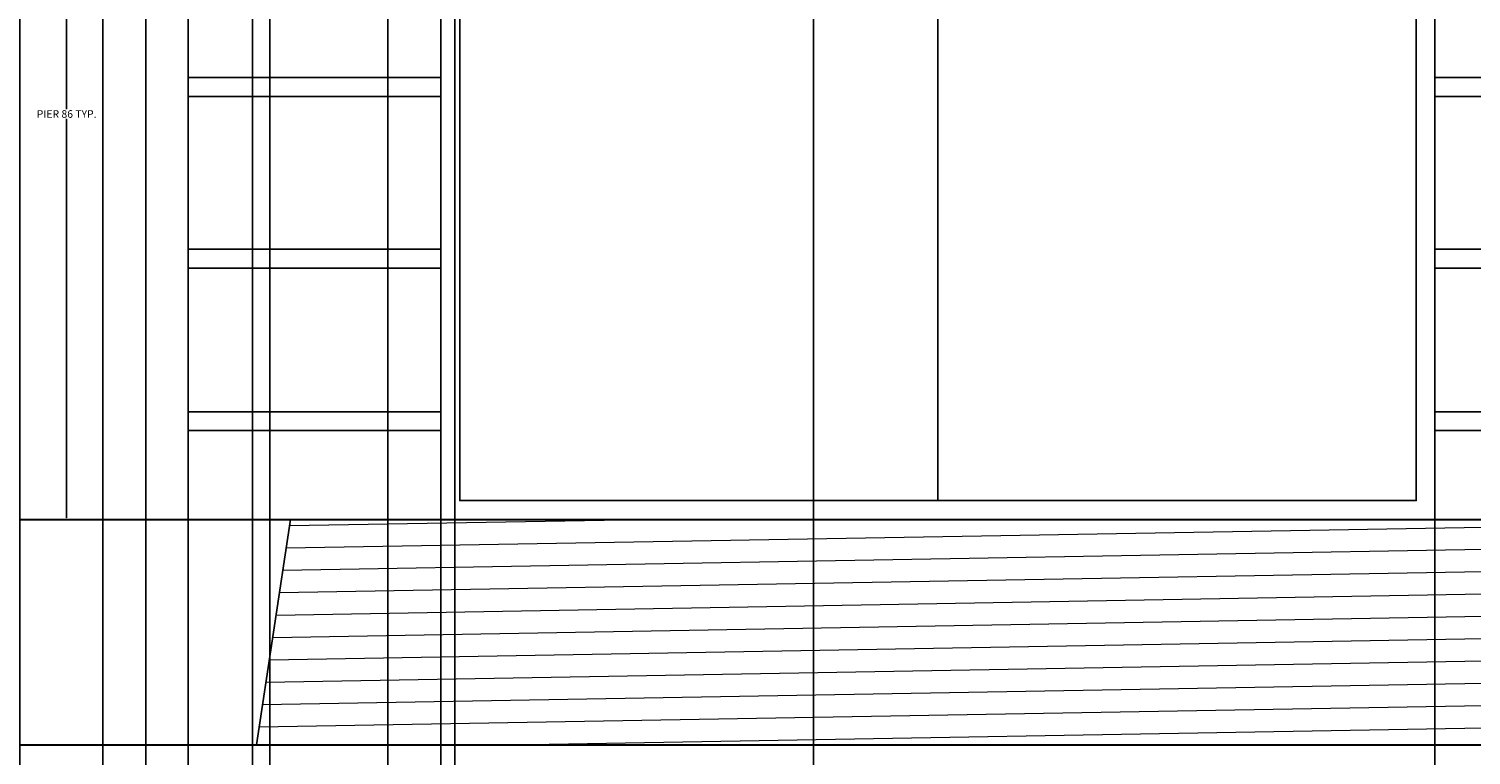
# Model space of a CAD drawing. Units: inches. Extents: x 69 to 650, y -16 to 573.
# Tile 7 of 26: x 345 to 499, y 63 to 140. Entities that reach past the tile are written whole.
import ezdxf

# ---------------------------------------------------------------- set-up
doc = ezdxf.new("R2010")
doc.units = ezdxf.units.IN
doc.header["$MEASUREMENT"] = 0
for name, color, linetype, lineweight in [('A-ANNO-DIMS', 2, 'Continuous', 18), ('A-COLS', 7, 'Continuous', 25), ('A-DOOR', 3, 'Continuous', 25), ('A-FLOR-PATT', 252, 'Continuous', 13), ('A-FLOR-STRS', 7, 'Continuous', 25), ('A-WALL-BASE', 7, 'Continuous', 30)]:
    doc.layers.add(name, color=color, linetype=linetype, lineweight=lineweight)
doc.styles.get("Standard").update_dxf_attribs({"font": 'arial.ttf'})
doc.dimstyles.get("Standard").update_dxf_attribs({"dimtxt": 0.8125, "dimasz": 0.18, "dimexe": 0.18, "dimexo": 0.0625, "dimgap": 0.09, "dimtad": 0, "dimtih": 1, "dimtoh": 1, "dimdec": 4, "dimzin": 0, "dimdsep": 46, "dimlunit": 4, "dimtxsty": 'Standard', "dimcen": 0.09, "dimadec": 0, "dimazin": 0, "dimtfac": 1, "dimtdec": 4, "dimtofl": 0, "dimtmove": 0, "dimatfit": 3, "dimfxl": 1, "dimtolj": 1, "dimtzin": 0, "dimarcsym": 0})

# ---------------------------------------------------------------- blocks, each defined once
blk = doc.blocks.new('PIER-PORTAL-BANDED')
for p, q in [((0, 0), (0, 86.34)), ((0, 86.34), (26.94, 86.34)), ((0, 66.41), (26.94, 66.41)), ((0, 64.41), (26.94, 64.41)), ((0, 47.05), (26.94, 47.05)), ((0, 45.05), (26.94, 45.05)), ((0, 28.76), (26.94, 28.76)), ((0, 26.76), (26.94, 26.76)), ((0, 11.45), (26.94, 11.45)), ((0, 9.45), (26.94, 9.45))]:
    blk.add_line(p, q)
blk = doc.blocks.new('*D15')
at = {"layer": 'A-ANNO-DIMS', "color": 0, "lineweight": -2, "transparency": 16777216}
for p, q in [((361.96, 174.27), (348.89, 174.27)), ((349.07, 174.09), (349.07, 131.6)), ((349.07, 88.11), (349.07, 130.59)), ((361.96, 87.93), (348.89, 87.93))]:
    blk.add_line(p, q, dxfattribs=at)
at = {"layer": 'A-ANNO-DIMS', "color": 0, "transparency": 16777216}
for points in [[(349.04, 174.09), (349.1, 174.09), (349.07, 174.27)], [(349.04, 88.11), (349.1, 88.11), (349.07, 87.93)]]:
    blk.add_solid(points, dxfattribs=at)
at = {"layer": 'Defpoints', "color": 0, "transparency": 16777216}
for p in [(349.07, 174.27), (362.02, 174.27), (362.02, 87.93)]:
    blk.add_point(p, dxfattribs=at)
at = {"layer": 'A-ANNO-DIMS', "color": 0, "transparency": 16777216, "insert": (349.07, 131.1), "char_height": 0.8125, "attachment_point": 5}
blk.add_mtext('\\A1;PIER 86 TYP.', dxfattribs=at)
blk = doc.blocks.new('*D19')
at = {"layer": 'A-ANNO-DIMS', "color": 0, "lineweight": -2, "transparency": 16777216}
for p, q in [((99.56, 471.72), (99.56, 572.74)), ((99.74, 572.56), (358.57, 572.56)), ((619.38, 572.56), (360.54, 572.56)), ((619.56, 87.99), (619.56, 572.74))]:
    blk.add_line(p, q, dxfattribs=at)
at = {"layer": 'A-ANNO-DIMS', "color": 0, "transparency": 16777216}
for points in [[(99.74, 572.59), (99.74, 572.53), (99.56, 572.56)], [(619.38, 572.59), (619.38, 572.53), (619.56, 572.56)]]:
    blk.add_solid(points, dxfattribs=at)
at = {"layer": 'Defpoints', "color": 0, "transparency": 16777216}
for p in [(619.56, 572.56), (99.56, 471.66), (619.56, 87.93)]:
    blk.add_point(p, dxfattribs=at)
at = {"layer": 'A-ANNO-DIMS', "color": 0, "transparency": 16777216, "insert": (359.56, 572.56), "char_height": 0.812, "attachment_point": 5}
blk.add_mtext('\\A1;520', dxfattribs=at)
blk = doc.blocks.new('*D30')
at = {"layer": 'A-ANNO-DIMS', "color": 0, "lineweight": -2, "transparency": 16777216}
for p, q in [((352.94, 174.2), (352.94, 35.35)), ((313.14, 87.92), (313.14, 35.35)), ((313.32, 35.53), (331.9, 35.53)), ((352.76, 35.53), (334.19, 35.53))]:
    blk.add_line(p, q, dxfattribs=at)
at = {"layer": 'A-ANNO-DIMS', "color": 0, "transparency": 16777216}
for points in [[(313.32, 35.56), (313.32, 35.5), (313.14, 35.53)], [(352.76, 35.56), (352.76, 35.5), (352.94, 35.53)]]:
    blk.add_solid(points, dxfattribs=at)
at = {"layer": 'Defpoints', "color": 0, "transparency": 16777216}
for p in [(352.94, 174.27), (313.14, 87.99), (352.94, 35.53)]:
    blk.add_point(p, dxfattribs=at)
at = {"layer": 'A-ANNO-DIMS', "color": 0, "transparency": 16777216, "insert": (333.04, 35.53), "char_height": 0.812, "attachment_point": 5}
blk.add_mtext('\\A1;39.8', dxfattribs=at)
blk = doc.blocks.new('*D31')
at = {"layer": 'A-ANNO-DIMS', "color": 0, "lineweight": -2, "transparency": 16777216}
for p, q in [((352.94, 174.2), (352.94, 35.35)), ((362.02, 87.87), (362.02, 35.35)), ((353.12, 35.53), (356.1, 35.53)), ((361.84, 35.53), (358.86, 35.53))]:
    blk.add_line(p, q, dxfattribs=at)
at = {"layer": 'A-ANNO-DIMS', "color": 0, "transparency": 16777216}
for points in [[(353.12, 35.56), (353.12, 35.5), (352.94, 35.53)], [(361.84, 35.56), (361.84, 35.5), (362.02, 35.53)]]:
    blk.add_solid(points, dxfattribs=at)
at = {"layer": 'Defpoints', "color": 0, "transparency": 16777216}
for p in [(352.94, 174.27), (362.02, 87.93), (362.02, 35.53)]:
    blk.add_point(p, dxfattribs=at)
at = {"layer": 'A-ANNO-DIMS', "color": 0, "transparency": 16777216, "insert": (357.48, 35.53), "char_height": 0.812, "attachment_point": 5}
blk.add_mtext('\\A1;9.081', dxfattribs=at)
blk = doc.blocks.new('*D32')
at = {"layer": 'A-ANNO-DIMS', "color": 0, "lineweight": -2, "transparency": 16777216}
for p, q in [((388.96, 87.87), (388.96, 35.35)), ((494.91, 87.87), (494.91, 35.35)), ((389.14, 35.53), (440.2, 35.53)), ((494.73, 35.53), (443.68, 35.53))]:
    blk.add_line(p, q, dxfattribs=at)
at = {"layer": 'A-ANNO-DIMS', "color": 0, "transparency": 16777216}
for points in [[(389.14, 35.56), (389.14, 35.5), (388.96, 35.53)], [(494.73, 35.56), (494.73, 35.5), (494.91, 35.53)]]:
    blk.add_solid(points, dxfattribs=at)
at = {"layer": 'Defpoints', "color": 0, "transparency": 16777216}
for p in [(388.96, 87.93), (494.91, 87.93), (494.91, 35.53)]:
    blk.add_point(p, dxfattribs=at)
at = {"layer": 'A-ANNO-DIMS', "color": 0, "transparency": 16777216, "insert": (441.94, 35.53), "char_height": 0.812, "attachment_point": 5}
blk.add_mtext('\\A1;105.95', dxfattribs=at)
blk = doc.blocks.new('*D38')
at = {"layer": 'A-ANNO-DIMS', "color": 0, "lineweight": -2, "transparency": 16777216}
for p, q in [((307.8, 384.84), (307.8, 35.35)), ((390.43, 384.84), (390.43, 35.35)), ((307.98, 35.53), (347.65, 35.53)), ((390.25, 35.53), (350.57, 35.53))]:
    blk.add_line(p, q, dxfattribs=at)
at = {"layer": 'A-ANNO-DIMS', "color": 0, "transparency": 16777216}
for points in [[(307.98, 35.56), (307.98, 35.5), (307.8, 35.53)], [(390.25, 35.56), (390.25, 35.5), (390.43, 35.53)]]:
    blk.add_solid(points, dxfattribs=at)
at = {"layer": 'Defpoints', "color": 0, "transparency": 16777216}
for p in [(307.8, 384.9), (390.43, 384.9), (390.43, 35.53)]:
    blk.add_point(p, dxfattribs=at)
at = {"layer": 'A-ANNO-DIMS', "color": 0, "transparency": 16777216, "insert": (349.11, 35.53), "char_height": 0.812, "attachment_point": 5}
blk.add_mtext('\\A1;82.63', dxfattribs=at)
blk = doc.blocks.new('*D39')
at = {"layer": 'A-ANNO-DIMS', "color": 0, "lineweight": -2, "transparency": 16777216}
for p, q in [((390.43, 384.84), (390.43, 35.35)), ((428.66, 372.93), (428.66, 35.35)), ((390.61, 35.53), (407.77, 35.53)), ((428.48, 35.53), (411.32, 35.53))]:
    blk.add_line(p, q, dxfattribs=at)
at = {"layer": 'A-ANNO-DIMS', "color": 0, "transparency": 16777216}
for points in [[(390.61, 35.56), (390.61, 35.5), (390.43, 35.53)], [(428.48, 35.56), (428.48, 35.5), (428.66, 35.53)]]:
    blk.add_solid(points, dxfattribs=at)
at = {"layer": 'Defpoints', "color": 0, "transparency": 16777216}
for p in [(390.43, 384.9), (428.66, 372.99), (428.66, 35.53)]:
    blk.add_point(p, dxfattribs=at)
at = {"layer": 'A-ANNO-DIMS', "color": 0, "transparency": 16777216, "insert": (409.55, 35.53), "char_height": 0.812, "attachment_point": 5}
blk.add_mtext('\\A1;38.236', dxfattribs=at)
blk = doc.blocks.new('*D65')
at = {"layer": 'A-ANNO-DIMS', "color": 0, "lineweight": -2, "transparency": 16777216}
for p, q in [((344.08, 393.8), (344.08, 35.35)), ((368.88, 393.8), (368.88, 35.35)), ((344.26, 35.53), (355.33, 35.53)), ((368.7, 35.53), (357.63, 35.53))]:
    blk.add_line(p, q, dxfattribs=at)
at = {"layer": 'A-ANNO-DIMS', "color": 0, "transparency": 16777216}
for points in [[(344.26, 35.56), (344.26, 35.5), (344.08, 35.53)], [(368.7, 35.56), (368.7, 35.5), (368.88, 35.53)]]:
    blk.add_solid(points, dxfattribs=at)
at = {"layer": 'Defpoints', "color": 0, "transparency": 16777216}
for p in [(344.08, 393.86), (368.88, 393.86), (368.88, 35.53)]:
    blk.add_point(p, dxfattribs=at)
at = {"layer": 'A-ANNO-DIMS', "color": 0, "transparency": 16777216, "insert": (356.48, 35.53), "char_height": 0.812, "attachment_point": 5}
blk.add_mtext('\\A1;24.8', dxfattribs=at)
blk = doc.blocks.new('*D69')
at = {"layer": 'A-ANNO-DIMS', "color": 0, "lineweight": -2, "transparency": 16777216}
for p, q in [((343.89, 263.46), (343.89, 35.35)), ((357.51, 263.46), (357.51, 35.35)), ((344.07, 35.53), (349.28, 35.53)), ((357.33, 35.53), (352.12, 35.53))]:
    blk.add_line(p, q, dxfattribs=at)
at = {"layer": 'A-ANNO-DIMS', "color": 0, "transparency": 16777216}
for points in [[(344.07, 35.56), (344.07, 35.5), (343.89, 35.53)], [(357.33, 35.56), (357.33, 35.5), (357.51, 35.53)]]:
    blk.add_solid(points, dxfattribs=at)
at = {"layer": 'Defpoints', "color": 0, "transparency": 16777216}
for p in [(343.89, 263.53), (357.51, 263.53), (357.51, 35.53)]:
    blk.add_point(p, dxfattribs=at)
at = {"layer": 'A-ANNO-DIMS', "color": 0, "transparency": 16777216, "insert": (350.7, 35.53), "char_height": 0.812, "attachment_point": 5}
blk.add_mtext('\\A1;13.62', dxfattribs=at)
blk = doc.blocks.new('*D70')
at = {"layer": 'A-ANNO-DIMS', "color": 0, "lineweight": -2, "transparency": 16777216}
for p, q in [((357.51, 263.46), (357.51, 35.35)), ((370.73, 263.46), (370.73, 35.35)), ((357.69, 35.53), (362.46, 35.53)), ((370.55, 35.53), (365.78, 35.53))]:
    blk.add_line(p, q, dxfattribs=at)
at = {"layer": 'A-ANNO-DIMS', "color": 0, "transparency": 16777216}
for points in [[(357.69, 35.56), (357.69, 35.5), (357.51, 35.53)], [(370.55, 35.56), (370.55, 35.5), (370.73, 35.53)]]:
    blk.add_solid(points, dxfattribs=at)
at = {"layer": 'Defpoints', "color": 0, "transparency": 16777216}
for p in [(357.51, 263.53), (370.73, 263.53), (370.73, 35.53)]:
    blk.add_point(p, dxfattribs=at)
at = {"layer": 'A-ANNO-DIMS', "color": 0, "transparency": 16777216, "insert": (364.12, 35.53), "char_height": 0.812, "attachment_point": 5}
blk.add_mtext('\\A1;13.221', dxfattribs=at)
blk = doc.blocks.new('*D71')
at = {"layer": 'A-ANNO-DIMS', "color": 0, "lineweight": -2, "transparency": 16777216}
for p, q in [((370.73, 263.46), (370.73, 35.35)), ((383.3, 263.46), (383.3, 35.35)), ((370.91, 35.53), (375.59, 35.53)), ((383.12, 35.53), (378.44, 35.53))]:
    blk.add_line(p, q, dxfattribs=at)
at = {"layer": 'A-ANNO-DIMS', "color": 0, "transparency": 16777216}
for points in [[(370.91, 35.56), (370.91, 35.5), (370.73, 35.53)], [(383.12, 35.56), (383.12, 35.5), (383.3, 35.53)]]:
    blk.add_solid(points, dxfattribs=at)
at = {"layer": 'Defpoints', "color": 0, "transparency": 16777216}
for p in [(370.73, 263.53), (383.3, 263.53), (383.3, 35.53)]:
    blk.add_point(p, dxfattribs=at)
at = {"layer": 'A-ANNO-DIMS', "color": 0, "transparency": 16777216, "insert": (377.02, 35.53), "char_height": 0.812, "attachment_point": 5}
blk.add_mtext('\\A1;12.57', dxfattribs=at)

msp = doc.modelspace()

# ---------------------------------------------------------------- hatches: boundary and pattern name
at = {"layer": 'A-FLOR-PATT'}
h = msp.add_hatch(dxfattribs=at)
h.set_pattern_fill('ANSI31', color=256, scale=19, angle=136)
h.paths.add_polyline_path([(506.932, 87.93), (463.7847, 87.93), (388.9646, 87.93), (372.9372, 87.93), (369.3072, 63.93), (463.7847, 63.93), (513.9402, 63.93)])

# ---------------------------------------------------------------- linework, layer by layer
at = {"layer": 'A-DOOR'}
msp.add_line((441.9398, 172.2666), (441.9398, 89.93), dxfattribs=at)
for points in [[(388.9646, 174.2666), (494.915, 174.2666), (494.915, 87.93), (388.9646, 87.93)], [(390.9646, 172.2666), (492.915, 172.2666), (492.915, 89.93), (390.9646, 89.93)]]:
    msp.add_lwpolyline(points, close=True, dxfattribs=at)
at = {"layer": 'A-FLOR-STRS'}
msp.add_lwpolyline([(372.9372, 87.93), (369.3072, 63.93)], dxfattribs=at)
at = {"layer": 'A-WALL-BASE'}
for p, q in [((99.556, 87.93), (463.7847, 87.93)), ((463.7847, 87.93), (557.8179, 87.93)), ((99.556, 63.93), (463.7847, 63.93)), ((463.7847, 63.93), (557.8179, 63.93))]:
    msp.add_line(p, q, dxfattribs=at)

# ---------------------------------------------------------------- block references
at = {"layer": 'A-COLS'}
msp.add_blockref('PIER-PORTAL-BANDED', (362.023, 87.93), dxfattribs=at)
at = {"layer": 'A-COLS', "extrusion": (0, 0, -1), "zscale": -1}
msp.add_blockref('PIER-PORTAL-BANDED', (-521.8566, 87.93), dxfattribs=at)

# ---------------------------------------------------------------- dimensions: what is measured, and where the dimension line sits
at = {"layer": 'A-ANNO-DIMS'}
for base, p1, p2, override, picture, middle in [((619.555, 572.5573), (99.556, 471.6595), (619.555, 87.93), {"dimdec": 0, "dimlfac": 1, "dimrnd": 0, "dimzin": 0, "dimdsep": 46, "dimlunit": 2}, '*D19', (359.5555, 572.5573)), ((368.881, 35.53), (344.0804, 393.8576), (368.881, 393.8576), {"dimdec": 1, "dimlfac": 1, "dimrnd": 0, "dimzin": 0, "dimdsep": 46, "dimlunit": 2}, '*D65', (356.4807, 35.53)), ((390.4291, 35.53), (307.7955, 384.8986), (390.4291, 384.8986), {"dimdec": 2, "dimlfac": 1, "dimrnd": 0, "dimzin": 0, "dimdsep": 46, "dimlunit": 2}, '*D38', (349.1123, 35.53)), ((428.6648, 35.53), (390.4291, 384.8986), (428.6648, 372.9907), {"dimdec": 3, "dimlfac": 1, "dimrnd": 0, "dimzin": 0, "dimdsep": 46, "dimlunit": 2}, '*D39', (409.547, 35.53)), ((357.5106, 35.53), (343.8902, 263.5253), (357.5106, 263.5253), {"dimdec": 2, "dimlfac": 1, "dimrnd": 0, "dimzin": 0, "dimdsep": 46, "dimlunit": 2}, '*D69', (350.7004, 35.53)), ((370.7319, 35.53), (357.5106, 263.5253), (370.7319, 263.5253), {"dimdec": 3, "dimlfac": 1, "dimrnd": 0, "dimzin": 0, "dimdsep": 46, "dimlunit": 2}, '*D70', (364.1213, 35.53)), ((383.3022, 35.53), (370.7319, 263.5253), (383.3022, 263.5253), {"dimdec": 2, "dimlfac": 1, "dimrnd": 0, "dimzin": 0, "dimdsep": 46, "dimlunit": 2}, '*D71', (377.0171, 35.53)), ((352.9415, 35.53), (313.1416, 87.985), (352.9415, 174.2666), {"dimdec": 1, "dimlfac": 1, "dimrnd": 0, "dimzin": 0, "dimdsep": 46, "dimlunit": 2}, '*D30', (333.0415, 35.53)), ((362.0229, 35.53), (352.9415, 174.2666), (362.0229, 87.93), {"dimdec": 3, "dimlfac": 1, "dimrnd": 0, "dimzin": 0, "dimdsep": 46, "dimlunit": 2}, '*D31', (357.4822, 35.53)), ((494.915, 35.53), (388.9646, 87.93), (494.915, 87.93), {"dimdec": 2, "dimlfac": 1, "dimrnd": 0, "dimzin": 0, "dimdsep": 46, "dimlunit": 2}, '*D32', (441.9398, 35.53))]:
    dim = msp.add_linear_dim(base=base, p1=p1, p2=p2, dimstyle='Standard', override=override, dxfattribs=at)
    dim.commit()
    dim.dimension.update_dxf_attribs({"geometry": picture, "text_midpoint": middle})
dim = msp.add_linear_dim(base=(349.0724, 174.2666), p1=(362.0229, 87.93), p2=(362.0229, 174.2666), angle=90, text='PIER <> TYP.', dimstyle='Standard', override={"dimdec": 0, "dimlfac": 1, "dimrnd": 0, "dimzin": 0, "dimdsep": 46, "dimlunit": 2}, dxfattribs=at)
dim.commit()
dim.dimension.update_dxf_attribs({"geometry": '*D15', "text_midpoint": (349.0724, 131.0983)})

doc.saveas('drawing.dxf')
